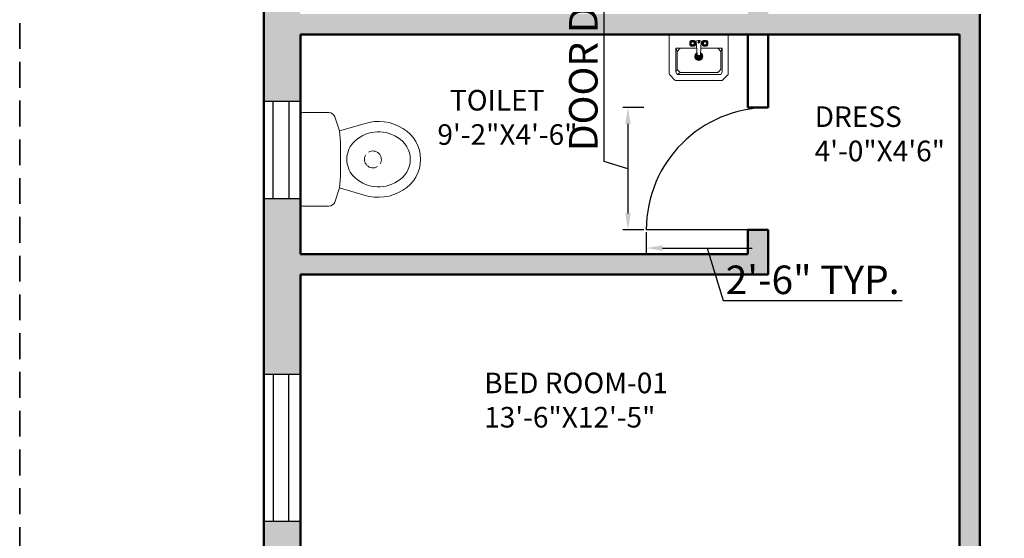
# Model space of a CAD drawing. Units: inches. Extents: x -7 to 1228, y -146 to 1091.
# Tile 48 of 88: x 0 to 242, y 658 to 786. Entities that reach past the tile are written whole.
import ezdxf

# ---------------------------------------------------------------- set-up
doc = ezdxf.new("R2010")
doc.units = ezdxf.units.IN
doc.linetypes.add('DASHED2', pattern=[9.525, 6.35, -3.175])
for name, color, linetype, lineweight in [('A-ANNO-DIMS', 2, 'Continuous', 18), ('A-AREA-IDEN', 7, 'Continuous', 18), ('A-DOOR', 4, 'Continuous', 25), ('A-FLOR-FIXT', 8, 'Continuous', 18), ('A-FURN', 8, 'Continuous', 18), ('A-GLAZ', 175, 'Continuous', 25), ('A-WALL', 7, 'Continuous', 50), ('A-WALL-PATT', 251, 'Continuous', 13), ('C-PROP', 1, 'DASHED2', 35)]:
    doc.layers.add(name, color=color, linetype=linetype, lineweight=lineweight)
doc.styles.get("Standard").update_dxf_attribs({"font": 'arial.ttf'})
doc.dimstyles.new('ISO-25', dxfattribs={"dimtxt": 7, "dimasz": 4, "dimexe": 1.25, "dimexo": 0.625, "dimtad": 1, "dimdec": 1, "dimlunit": 3, "dimtxsty": 'Standard', "dimcen": 2.5, "dimadec": 0, "dimazin": 0, "dimtfac": 1, "dimtdec": 1, "dimtmove": 1, "dimatfit": 3, "dimfxl": 1, "dimarcsym": 0})

# ---------------------------------------------------------------- blocks, each defined once
blk = doc.blocks.new('A$C7B5C7CD4')
at = {"ltscale": 20}
for p, q in [((0.243, 0.625), (0.011, 0.625)), ((0.243, 0.625), (0.475, 0.625)), ((0, 0.614), (0, 0.4765)), ((0.486, 0.614), (0.486, 0.4765)), ((0.0212, 0.4467), (0.0946, 0.4214)), ((0.0946, 0.4214), (0.0576, 0.293)), ((0.0946, 0.4214), (0.1544, 0.4173)), ((0.3316, 0.4173), (0.1544, 0.4173)), ((0.3914, 0.4214), (0.3316, 0.4173)), ((0.4648, 0.4467), (0.3914, 0.4214)), ((0.3914, 0.4214), (0.4284, 0.293))]:
    blk.add_line(p, q, dxfattribs=at)
for centre, radius, start, end in [((0.011, 0.614), 0.011, 90, 180), ((0.475, 0.614), 0.011, 0, 90), ((0.0315, 0.4765), 0.0315, 180, 251), ((0.4545, 0.4765), 0.0315, 289, 0), ((0.24, 0.2602), 0.123, 88.6158, 131.7414), ((0.246, 0.2602), 0.123, 48.2586, 91.3842), ((0.2796, 0.219), 0.18, 132.4207, 213.289), ((0.2064, 0.219), 0.18, 326.711, 47.5793), ((0.2796, 0.219), 0.234, 161.5846, 212.8753), ((0.2064, 0.219), 0.234, 327.1247, 18.4154), ((0.243, 0.185), 0.131, 209.6292, 270), ((0.243, 0.185), 0.131, 270, 330.3708), ((0.243, 0.185), 0.185, 210.1745, 270), ((0.243, 0.185), 0.185, 270, 329.8255)]:
    blk.add_arc(centre, radius, start, end, dxfattribs=at)
for start, end in [(58.1785, 211.8215), (238.1785, 31.8215)]:
    blk.add_arc((0.2426, 0.2481), 0.0439, start, end)
blk = doc.blocks.new('A$C4CB854FF')
for p, q in [((0, 0.3675), (0, 0.0552)), ((0.4725, 0.38), (0.0125, 0.38)), ((0.1787, 0.329), (0.2034, 0.329)), ((0.2337, 0.329), (0.2502, 0.329)), ((0.3052, 0.329), (0.2804, 0.329)), ((0.485, 0.0552), (0.485, 0.3675)), ((0.05, 0.265), (0.2247, 0.265)), ((0.06, 0.24), (0.05, 0.265)), ((0.05, 0.07), (0.05, 0.265)), ((0.085, 0.265), (0.06, 0.24)), ((0.1677, 0.2932), (0.1677, 0.318)), ((0.1745, 0.2919), (0.1745, 0.3194)), ((0.1773, 0.3221), (0.2048, 0.3221)), ((0.2048, 0.2891), (0.1773, 0.2891)), ((0.2034, 0.2822), (0.1787, 0.2822)), ((0.2075, 0.3194), (0.2075, 0.2919)), ((0.2144, 0.318), (0.2144, 0.2932)), ((0.2279, 0.2104), (0.2213, 0.3235)), ((0.2625, 0.3235), (0.256, 0.2104)), ((0.2591, 0.265), (0.43, 0.265)), ((0.2694, 0.318), (0.2694, 0.2932)), ((0.2763, 0.3194), (0.2763, 0.2919)), ((0.3065, 0.3221), (0.279, 0.3221)), ((0.279, 0.2891), (0.3065, 0.2891)), ((0.2804, 0.2822), (0.3052, 0.2822)), ((0.3093, 0.2919), (0.3093, 0.3194)), ((0.3162, 0.2932), (0.3162, 0.318)), ((0.395, 0.265), (0.42, 0.24)), ((0.42, 0.24), (0.43, 0.265)), ((0.43, 0.07), (0.43, 0.265)), ((0.06, 0.24), (0.06, 0.09)), ((0.2152, 0.1984), (0.2694, 0.1984)), ((0.2297, 0.2066), (0.2165, 0.2066)), ((0.2681, 0.1901), (0.2165, 0.1901)), ((0.2272, 0.2149), (0.2208, 0.2149)), ((0.2638, 0.1819), (0.2208, 0.1819)), ((0.2533, 0.1736), (0.2313, 0.1736)), ((0.2505, 0.2052), (0.2334, 0.2052)), ((0.2681, 0.2066), (0.2541, 0.2066)), ((0.2638, 0.2149), (0.2566, 0.2149)), ((0.42, 0.24), (0.42, 0.09)), ((0.06, 0.09), (0.085, 0.065)), ((0.42, 0.09), (0.395, 0.065)), ((0.42, 0.09), (0.43, 0.07)), ((0.0037, 0.0463), (0.0463, 0.0037)), ((0.05, 0.07), (0.06, 0.05)), ((0.42, 0.05), (0.06, 0.05)), ((0.085, 0.065), (0.395, 0.065)), ((0.395, 0.065), (0.42, 0.05)), ((0.43, 0.07), (0.42, 0.05)), ((0.4387, 0.0037), (0.4813, 0.0463)), ((0.0552, 0), (0.4298, 0))]:
    blk.add_line(p, q)
for centre, radius in [((0.191, 0.3056), 0.0165), ((0.191, 0.3056), 0.0127), ((0.2419, 0.3152), 0.00688), ((0.2419, 0.3152), 0.00344), ((0.2928, 0.3056), 0.0165), ((0.2928, 0.3056), 0.0127)]:
    blk.add_circle(centre, radius)
for centre, radius, start, end in [((0.0125, 0.3675), 0.0125, 90, 180), ((0.1787, 0.318), 0.011, 90, 180), ((0.2034, 0.318), 0.011, 0, 90), ((0.2329, 0.314), 0.015, 87.19754, 140.72744), ((0.2509, 0.314), 0.015, 39.27256, 92.80246), ((0.2804, 0.318), 0.011, 90, 180), ((0.3052, 0.318), 0.011, 0, 90), ((0.4725, 0.3675), 0.0125, 0, 90), ((0.1787, 0.2932), 0.011, 180, 270), ((0.1773, 0.3194), 0.00275, 90, 180), ((0.1773, 0.2919), 0.00275, 180, 270), ((0.2034, 0.2932), 0.011, 270, 0), ((0.2048, 0.3194), 0.00275, 360, 90), ((0.2048, 0.2919), 0.00275, 270, 0), ((0.2804, 0.2932), 0.011, 180, 270), ((0.279, 0.3194), 0.00275, 90, 180), ((0.279, 0.2919), 0.00275, 180, 270), ((0.3052, 0.2932), 0.011, 270, 360), ((0.3065, 0.3194), 0.00275, 360, 90), ((0.3065, 0.2919), 0.00275, 270, 0), ((0.2423, 0.1984), 0.033, 118.68833, 62.86857), ((0.2423, 0.1984), 0.0271, 124.77581, 57.22467), ((0.2334, 0.2107), 0.0055, 183.3274, 270), ((0.2505, 0.2107), 0.0055, 270, 356.6726), ((0.0125, 0.0552), 0.0125, 180, 225), ((0.0552, 0.0125), 0.0125, 225, 270), ((0.4298, 0.0125), 0.0125, 270, 315), ((0.4725, 0.0552), 0.0125, 315, 0)]:
    blk.add_arc(centre, radius, start, end)
blk = doc.blocks.new('WIN-36')
for p, q in [((0, 36), (0, 0)), ((9, 36), (0, 36)), ((2.34, 36), (2.34, 0)), ((6.14, 0), (6.14, 36)), ((9, 0), (9, 36)), ((0, 0), (9, 0)), ((2.34, 0), (6.14, 0))]:
    blk.add_line(p, q)
blk = doc.blocks.new('WIN-24')
for p, q in [((0, 0), (0, 24)), ((0, 24), (9, 24)), ((2.34, 0), (2.34, 24)), ((2.34, 24), (6.14, 24)), ((6.14, 24), (6.14, 0)), ((9, 24), (9, 0)), ((9, 0), (0, 0))]:
    blk.add_line(p, q)
blk = doc.blocks.new('DOOR-750')
blk.add_line((30, 30), (30, 0))
blk.add_arc((30, 30), 30, 180, 270)
blk = doc.blocks.new('*D46')
at = {"layer": 'A-ANNO-DIMS', "color": 0, "lineweight": -2, "transparency": 16777216}
for p, q in [((143.69, 750.74), (143.69, 841.58)), ((153.38, 764), (148.25, 764)), ((149.5, 760), (149.5, 738)), ((149.5, 749), (143.69, 750.74)), ((153.38, 734), (148.25, 734))]:
    blk.add_line(p, q, dxfattribs=at)
at = {"layer": 'A-ANNO-DIMS', "color": 0, "transparency": 16777216}
for points in [[(148.83, 760), (150.17, 760), (149.5, 764)], [(148.83, 738), (150.17, 738), (149.5, 734)]]:
    blk.add_solid(points, dxfattribs=at)
at = {"layer": 'Defpoints', "color": 0, "transparency": 16777216}
for p in [(154, 764), (149.5, 734), (154, 734)]:
    blk.add_point(p, dxfattribs=at)
at = {"layer": 'A-ANNO-DIMS', "color": 0, "transparency": 16777216, "insert": (139.44, 796.16), "char_height": 7, "attachment_point": 5, "rotation": 90}
blk.add_mtext('DOOR D2 2\'-6" TYP.', dxfattribs=at)
blk = doc.blocks.new('*D47')
at = {"layer": 'A-ANNO-DIMS', "color": 0, "lineweight": -2, "transparency": 16777216}
for p, q in [((154, 733.38), (154, 728.25)), ((184, 733.38), (184, 728.25)), ((158, 729.5), (180, 729.5)), ((169, 729.5), (172.87, 716.59)), ((172.87, 716.59), (216.91, 716.59))]:
    blk.add_line(p, q, dxfattribs=at)
at = {"layer": 'A-ANNO-DIMS', "color": 0, "transparency": 16777216}
for points in [[(158, 730.17), (158, 728.83), (154, 729.5)], [(180, 730.17), (180, 728.83), (184, 729.5)]]:
    blk.add_solid(points, dxfattribs=at)
at = {"layer": 'Defpoints', "color": 0, "transparency": 16777216}
for p in [(154, 734), (184, 734), (184, 729.5)]:
    blk.add_point(p, dxfattribs=at)
at = {"layer": 'A-ANNO-DIMS', "color": 0, "transparency": 16777216, "insert": (194.89, 720.79), "char_height": 7, "attachment_point": 5}
blk.add_mtext('2\'-6" TYP.', dxfattribs=at)

msp = doc.modelspace()

# ---------------------------------------------------------------- hatches: boundary and pattern name
at = {"layer": 'A-WALL-PATT'}
h = msp.add_hatch(color=256, dxfattribs=at)
h.dxf.hatch_style = 1
h.paths.add_polyline_path([(69, 568), (60, 568), (60, 493), (63.29, 493), (69, 493)])
h.paths.add_polyline_path([(69, 662.41), (60, 662.41), (60, 586), (69, 586)], flags=17)
h.paths.add_polyline_path([(69, 723), (184, 723), (184, 734), (179, 734), (179, 728), (69, 728), (69, 741.62), (60, 741.62), (60, 698.41), (69, 698.41)], flags=17)
h.paths.add_polyline_path([(69, 782), (231, 782), (231, 728), (231, 723), (231, 586), (236, 586), (236, 787), (69, 787), (69, 800.13), (60, 800.13), (60, 765.62), (69, 765.62)])
h.paths.add_polyline_path([(184, 842), (189, 842), (189, 848), (173, 848), (173, 842), (179, 842), (179, 787), (184, 787)])
h.paths.add_polyline_path([(118.22, 69), (69, 69), (69, 60), (118.22, 60)])
h.paths.add_polyline_path([(227, 69), (154.22, 69), (154.22, 60), (227, 60)])
h.paths.add_polyline_path([(236, 60), (232.71, 60), (227, 60), (227, 36), (236, 36)])
h.paths.add_polyline_path([(389, 60), (380, 60), (380, 36), (389, 36)])
h.paths.add_polyline_path([(384, 181), (380, 181), (380, 115), (380, 78), (384, 78)])
h.paths.add_polyline_path([(380, 115), (334.55, 115), (334.55, 109), (380, 109)])
h.paths.add_polyline_path([(274.55, 115), (236, 115), (236, 201), (232.71, 201), (231, 201), (231, 78), (236, 78), (236, 109), (274.55, 109)])
h.paths.add_polyline_path([(69, 123), (60, 123), (60, 78), (69, 78)])
h.paths.add_polyline_path([(69, 201), (60, 201), (60, 159), (69, 159)])
h.paths.add_polyline_path([(143, 219), (69, 219), (69, 213), (143, 213)], flags=17)
h.paths.add_polyline_path([(189, 219), (184, 219), (184, 274), (231, 274), (231, 219), (236, 219), (236, 279), (184, 279), (184, 297), (179, 297), (179, 279), (69, 279), (69, 290.91), (60, 290.91), (60, 262.18), (69, 262.18), (69, 274), (179, 274), (179, 219), (173, 219), (173, 213), (189, 213)])
h.paths.add_polyline_path([(69, 238.18), (60, 238.18), (60, 219), (69, 219)], flags=17)
h.paths.add_polyline_path([(69, 333), (60, 333), (60, 314.91), (69, 314.91), (69, 316.96)])
h.paths.add_polyline_path([(190, 338), (184, 338), (69, 338), (69, 333), (179, 333), (179, 327), (184, 327), (184, 333.02), (190, 333.05)])
h.paths.add_polyline_path([(69, 386.81), (60, 386.81), (60, 351), (69, 351)])
h.paths.add_polyline_path([(69, 475), (60, 475), (60, 422.81), (69, 422.81)])
h.paths.add_polyline_path([(236, 475), (231, 475), (231, 351.24), (236, 351.24)])
h.paths.add_polyline_path([(384, 475), (380, 475), (380, 362), (384, 362)])
h.paths.add_polyline_path([(547, 307), (439, 307), (439, 356), (445, 356), (445, 362), (433, 362), (433, 307), (380, 307), (380, 244), (380, 241), (384, 241), (384, 301), (433, 301), (433, 277), (439, 277), (439, 301), (547, 301)])
h.paths.add_polyline_path([(547, 241), (439, 241), (439, 247), (433, 247), (433, 235), (547, 235)])
h.paths.add_polyline_path([(450, 69), (440.29, 69), (424.89, 69), (389, 69), (389, 60), (450, 60)])
h.paths.add_polyline_path([(547, 69), (486, 69), (486, 60), (547, 60)])
h.paths.add_polyline_path([(556, 148.27), (547, 148.27), (547, 78), (556, 78)])
h.paths.add_polyline_path([(556, 223), (547, 223), (547, 195), (547, 184.27), (556, 184.27)])
h.paths.add_polyline_path([(556, 311.19), (547, 311.19), (547, 273.08), (556, 273.08)])
h.paths.add_polyline_path([(556, 344), (552.71, 344), (547, 344), (547, 335.19), (556, 335.19)])
h.paths.add_polyline_path([(556, 249.08), (547, 249.08), (547, 241), (556, 241)])
h.paths.add_polyline_path([(547, 362), (475, 362), (475, 356), (547, 356)], flags=0)
h.paths.add_polyline_path([(556, 399.62), (547, 399.62), (547, 362), (556, 362)])
h.paths.add_polyline_path([(556, 475), (547, 475), (547, 435.62), (556, 435.62)])
h.paths.add_polyline_path([(547, 493), (389, 493), (389, 487), (547, 487)])
h.paths.add_polyline_path([(380, 493), (278, 493), (278, 487), (380, 487)])
h.paths.add_polyline_path([(227, 493), (69, 493), (69, 487), (227, 487)])
h.paths.add_polyline_path([(643, 122.44), (634, 122.44), (634, 78), (643, 78)])
h.paths.add_polyline_path([(702.5, 69), (692.79, 69), (677.39, 69), (643, 69), (643, 60), (702.5, 60)])
h.paths.add_polyline_path([(798, 69), (738.5, 69), (738.5, 60), (798, 60)])
h.paths.add_polyline_path([(807, 60), (803.71, 60), (798, 60), (798, 36), (807, 36)])
h.paths.add_polyline_path([(807, 109), (846.75, 109), (846.75, 115), (807, 115), (807, 159), (802, 159), (802, 78), (807, 78)])
h.paths.add_polyline_path([(807, 201), (802, 201), (802, 195), (807, 195)])
h.paths.add_polyline_path([(643, 201), (634, 201), (634, 158.44), (643, 158.44)])
h.paths.add_polyline_path([(756, 225), (751, 225), (751, 219), (643, 219), (643, 213), (756, 213)])
h.paths.add_polyline_path([(643, 240.85), (634, 240.85), (634, 219), (643, 219)])
h.paths.add_polyline_path([(643, 274), (643, 288.63), (634, 288.63), (634, 264.85), (643, 264.85)])
h.paths.add_polyline_path([(802, 279), (756, 279), (756, 297), (751, 297), (751, 279), (643, 279), (643, 274), (751, 274), (751, 255), (756, 255), (756, 274), (802, 274)])
h.paths.add_polyline_path([(807, 333), (803.71, 333), (802, 333), (802, 279), (802, 274), (802, 219), (807, 219)])
h.paths.add_polyline_path([(956, 182), (951, 182), (951, 115), (906.75, 115), (906.75, 109), (951, 109), (951, 78), (956, 78)])
h.paths.add_polyline_path([(960, 60), (951, 60), (951, 36), (960, 36)])
h.paths.add_polyline_path([(1021, 69), (1005.78, 69), (960, 69), (960, 60), (1021, 60)])
h.paths.add_polyline_path([(956, 224), (951, 224), (951, 218), (956, 218)])
h.paths.add_polyline_path([(956, 302), (1004, 302), (1004, 278), (1010, 278), (1010, 302), (1118, 302), (1118, 290.81), (1127, 290.81), (1127, 326.97), (1118, 326.97), (1118, 320.97), (1118, 307), (1010, 307), (1010, 356), (1016, 356), (1016, 362), (1004, 362), (1004, 307), (951, 307), (951, 244), (951, 242), (954.29, 242), (956, 242)])
h.paths.add_polyline_path([(643, 333), (634, 333), (634, 312.63), (643, 312.63), (643, 316.96)])
h.paths.add_polyline_path([(756, 338), (643, 338), (643, 333), (751, 333), (751, 327), (756, 327)])
h.paths.add_polyline_path([(643, 388), (634, 388), (634, 351), (643, 351)])
h.paths.add_polyline_path([(807, 357), (802, 357), (802, 351), (807, 351)])
h.paths.add_polyline_path([(807, 475), (802, 475), (802, 393), (807, 393)])
h.paths.add_polyline_path([(643, 475), (634, 475), (634, 424), (643, 424)])
h.paths.add_polyline_path([(798, 493), (643, 493), (643, 487), (798, 487)])
h.paths.add_polyline_path([(634, 493), (556, 493), (556, 487), (634, 487)])
h.paths.add_polyline_path([(813, 493), (807, 493), (807, 487), (813, 487)])
h.paths.add_polyline_path([(951, 493), (849, 493), (849, 487), (951, 487)])
h.paths.add_polyline_path([(956, 484), (951, 484), (951, 374), (956, 374)])
h.paths.add_polyline_path([(1109, 493), (969, 493), (969, 487), (1109, 487)])
h.paths.add_polyline_path([(1127, 484), (1118, 484), (1118, 450.64), (1127, 450.64)])
h.paths.add_polyline_path([(1127, 414.64), (1118, 414.64), (1118, 365), (1127, 365)])
h.paths.add_polyline_path([(1109, 362), (1046, 362), (1046, 356), (1109, 356)], flags=17)
h.paths.add_polyline_path([(1127, 356), (1123.45, 356), (1118, 356), (1118, 350.97), (1127, 350.97)], flags=0)
h.paths.add_polyline_path([(1127, 266.81), (1118, 266.81), (1118, 262.36), (1118, 242), (1127, 242)], flags=17)
h.paths.add_polyline_path([(1118, 242), (1010, 242), (1010, 248), (1004, 248), (1004, 237), (1118, 237)])
h.paths.add_polyline_path([(1127, 224), (1118, 224), (1118, 170), (1127, 170)])
h.paths.add_polyline_path([(1127, 134), (1118, 134), (1118, 78), (1127, 78)])
h.paths.add_polyline_path([(1118, 69), (1057, 69), (1057, 60), (1118, 60)])
h.paths.add_polyline_path([(227, 571.55), (227, 574), (69, 574), (69, 568), (227, 568)])
h.paths.add_polyline_path([(380, 571.55), (380, 574), (278, 574), (278, 568), (380, 568)])
h.paths.add_polyline_path([(242, 574), (236, 574), (236, 568), (242, 568)])
h.paths.add_polyline_path([(547, 571.55), (547, 574), (389, 574), (389, 568), (547, 568)])
h.paths.add_polyline_path([(384, 733), (380, 733), (380, 586), (384, 586)])
h.paths.add_polyline_path([(556, 646), (634, 646), (634, 655), (547, 655), (547, 586), (556, 586)])
h.paths.add_polyline_path([(634, 574), (556, 574), (556, 568), (634, 568)])
h.paths.add_polyline_path([(643, 655), (634, 655), (634, 586), (643, 586)])
h.paths.add_polyline_path([(798, 574), (643, 574), (643, 568), (798, 568)])
h.paths.add_polyline_path([(643, 663.85), (634, 663.85), (634, 655), (643, 655)])
h.paths.add_polyline_path([(556, 676.97), (547, 676.97), (547, 655), (556, 655)])
h.paths.add_polyline_path([(556, 733), (547, 733), (547, 712.97), (556, 712.97)])
h.paths.add_polyline_path([(643, 710), (634, 710), (634, 699.85), (643, 699.85)])
h.paths.add_polyline_path([(807, 668), (802, 668), (802, 586), (807, 586)])
h.paths.add_polyline_path([(951, 574), (849, 574), (849, 568), (951, 568)])
h.paths.add_polyline_path([(956, 691), (951, 691), (951, 577), (956, 577)])
h.paths.add_polyline_path([(1109, 574), (969, 574), (969, 568), (1109, 568)])
h.paths.add_polyline_path([(1127, 643.4), (1118, 643.4), (1118, 577), (1127, 577)])
h.paths.add_polyline_path([(1127, 568), (1123.45, 568), (1118, 568), (1118, 493), (1127, 493)])
h.paths.add_polyline_path([(1127, 733), (1118, 733), (1118, 679.4), (1127, 679.4)])
h.paths.add_polyline_path([(1127, 777.35), (1118, 777.35), (1118, 770.04), (1118, 751), (1127, 751)], flags=17)
h.paths.add_polyline_path([(1118, 751), (1010, 751), (1010, 757), (1004, 757), (1004, 745), (1118, 745)])
h.paths.add_polyline_path([(956, 811), (1004, 811), (1004, 787), (1010, 787), (1010, 811), (1017.87, 811), (1017.87, 811.63, -0.414214), (1018.25, 812), (1031.98, 812, -0.414214), (1032.35, 811.63), (1032.35, 811), (1118, 811), (1118, 801.35), (1127, 801.35), (1127, 834.69), (1118, 834.69), (1118, 830.24), (1118, 817), (1010, 817), (1010, 866), (1016, 866), (1016, 872), (1004, 872), (1004, 817), (956, 817), (956, 866), (951, 866), (951, 751), (954.29, 751), (956, 751)])
h.paths.add_polyline_path([(1118, 872), (1046, 872), (1046, 866), (1118, 866)], flags=17)
h.paths.add_polyline_path([(1127, 924.71), (1118, 924.71), (1118, 884), (1127, 884)])
h.paths.add_polyline_path([(1127, 866), (1123.71, 866), (1118, 866), (1118, 858.69), (1127, 858.69)], flags=17)
h.paths.add_polyline_path([(956, 983), (951, 983), (951, 952), (807, 952), (807, 983), (802, 983), (802, 902), (807, 902), (807, 946), (951, 946), (951, 884), (956, 884)])
h.paths.add_polyline_path([(807, 842), (802, 842), (802, 787), (756, 787), (756, 806), (751, 806), (751, 787), (643, 787), (643, 782), (751, 782), (751, 764), (756, 764), (756, 782), (802, 782), (802, 728), (807, 728)])
h.paths.add_polyline_path([(756, 848), (643, 848), (643, 842), (751, 842), (751, 836), (756, 836)])
h.paths.add_polyline_path([(756, 734), (751, 734), (751, 728), (643, 728), (643, 723), (756, 723)])
h.paths.add_polyline_path([(643, 749.79), (634, 749.79), (634, 728), (637.29, 728), (643, 728)])
h.paths.add_polyline_path([(643, 805.41), (634, 805.41), (634, 773.79), (643, 773.79)])
h.paths.add_polyline_path([(643, 896.66), (634, 896.66), (634, 860), (637.29, 860), (643, 860)])
h.paths.add_polyline_path([(643, 842), (634, 842), (634, 829.41), (643, 829.41)])
h.paths.add_polyline_path([(643, 983), (634, 983), (634, 932.66), (643, 932.66)])
h.paths.add_polyline_path([(1127, 983), (1118, 983), (1118, 960.71), (1127, 960.71)])
h.paths.add_polyline_path([(1118, 1001), (1077.53, 1001), (1077.53, 992), (1118, 992)])
h.paths.add_polyline_path([(1041.53, 1001), (960, 1001), (960, 992), (1041.53, 992)])
h.paths.add_polyline_path([(960, 1025), (951, 1025), (951, 1001), (954.29, 1001), (960, 1001)])
h.paths.add_polyline_path([(807, 1025), (798, 1025), (798, 1001), (807, 1001)])
h.paths.add_polyline_path([(798, 1001), (738.5, 1001), (738.5, 992), (798, 992)])
h.paths.add_polyline_path([(702.5, 1001), (643, 1001), (643, 992), (702.5, 992)])
h.paths.add_polyline_path([(547, 1001), (499.11, 1001), (499.11, 992), (547, 992)])
h.paths.add_polyline_path([(463.11, 1001), (389, 1001), (389, 992), (463.11, 992)])
h.paths.add_polyline_path([(389, 1025), (380, 1025), (380, 1022), (380, 1001), (383.29, 1001), (389, 1001)])
h.paths.add_polyline_path([(236, 1025), (227, 1025), (227, 1001), (236, 1001)])
h.paths.add_polyline_path([(236, 983), (231, 983), (231, 860), (236, 860)])
h.paths.add_polyline_path([(274.55, 952), (236, 952), (236, 946), (274.55, 946)])
h.paths.add_polyline_path([(380, 952), (334.55, 952), (334.55, 946), (380, 946)])
h.paths.add_polyline_path([(384, 983), (380, 983), (380, 884), (383.29, 884), (384, 884)])
h.paths.add_polyline_path([(227, 1001), (155.01, 1001), (155.01, 992), (162.87, 992), (227, 992)])
h.paths.add_polyline_path([(119.01, 1001), (69, 1001), (69, 992), (119.01, 992)])
h.paths.add_polyline_path([(69, 983), (60, 983), (60, 922.99), (69, 922.99)])
h.paths.add_polyline_path([(69, 886.99), (60, 886.99), (60, 860), (63.29, 860), (69, 860)])
h.paths.add_polyline_path([(143, 848), (69, 848), (69, 842), (143, 842)])

# ---------------------------------------------------------------- linework, layer by layer
at = {"layer": 'A-WALL'}
for p, q in [((60, 1001), (60, 60)), ((236, 787), (236, 574)), ((231, 782), (69, 782)), ((69, 782), (69, 728)), ((179, 782), (179, 764)), ((184, 782), (184, 764)), ((231, 782), (231, 728)), ((184, 764), (179, 764)), ((184, 734), (179, 734)), ((179, 734), (179, 728)), ((184, 734), (184, 723)), ((179, 728), (69, 728)), ((231, 723), (231, 728)), ((184, 723), (69, 723)), ((69, 723), (69, 574)), ((231, 723), (231, 574))]:
    msp.add_line(p, q, dxfattribs=at)
at = {"layer": 'C-PROP'}
msp.add_line((0, 1061), (0, 0), dxfattribs=at)

# ---------------------------------------------------------------- block references
at = {"layer": 'A-DOOR', "rotation": 269.9999999999998}
msp.add_blockref('DOOR-750', (154, 764), dxfattribs=at)
at = {"layer": 'A-FLOR-FIXT', "xscale": 47.26153857112405, "yscale": 47.26153857112405, "zscale": 47.26153857112405, "rotation": 90}
msp.add_blockref('A$C7B5C7CD4', (98.54, 739.81), dxfattribs=at)
at = {"layer": 'A-FURN', "xscale": -29.84864686937646, "yscale": 29.84864686937646, "zscale": 29.84864686937646}
msp.add_blockref('A$C4CB854FF', (174.13, 770.66), dxfattribs=at)
at = {"layer": 'A-GLAZ'}
for name, p in [('WIN-24', (60, 741.62)), ('WIN-36', (60, 662.4))]:
    msp.add_blockref(name, p, dxfattribs=at)

# ---------------------------------------------------------------- texts
at = {"layer": 'A-AREA-IDEN', "attachment_point": 1}
for s, insert, char_height in [('  TOILET\\P9\'-2"X4\'-6"', (102.66, 768.35), 5.0568), ('DRESS\\P4\'-0"X4\'6"', (195.39, 764.31), 5.057), ('BED ROOM-01\\P13\'-6"X12\'-5"', (114.16, 698.89), 5.0568)]:
    msp.add_mtext_dynamic_manual_height_columns(s, width=137.2821, gutter_width=25.28, heights=[0], dxfattribs=dict(at, insert=insert, char_height=char_height))

# ---------------------------------------------------------------- dimensions: what is measured, and where the dimension line sits
at = {"layer": 'A-ANNO-DIMS'}
dim = msp.add_linear_dim(base=(149.5, 734), p1=(154, 764), p2=(154, 734), angle=270, text='DOOR D2 <> TYP.', dimstyle='ISO-25', override={"dimdec": 1, "dimlfac": 1, "dimrnd": 0, "dimzin": 1, "dimdsep": 46, "dimlunit": 4, "dimfrac": 2}, dxfattribs=at)
dim.commit()
dim.dimension.update_dxf_attribs({"geometry": '*D46', "text_midpoint": (139.44, 751.37)})
dim = msp.add_linear_dim(base=(184, 729.5), p1=(154, 734), p2=(184, 734), text='<> TYP.', dimstyle='ISO-25', override={"dimdec": 1, "dimlfac": 1, "dimrnd": 0, "dimzin": 1, "dimdsep": 46, "dimlunit": 4, "dimfrac": 2}, dxfattribs=at)
dim.commit()
dim.dimension.update_dxf_attribs({"geometry": '*D47', "text_midpoint": (173.5, 720.79)})

doc.saveas('drawing.dxf')
